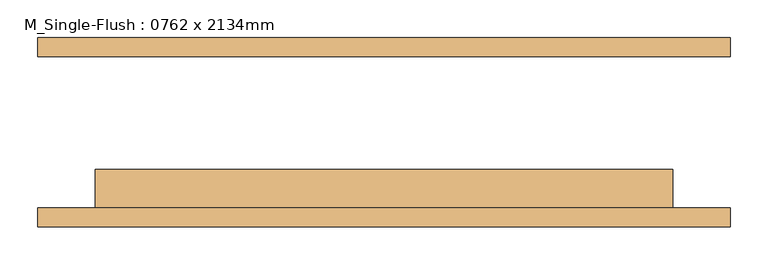
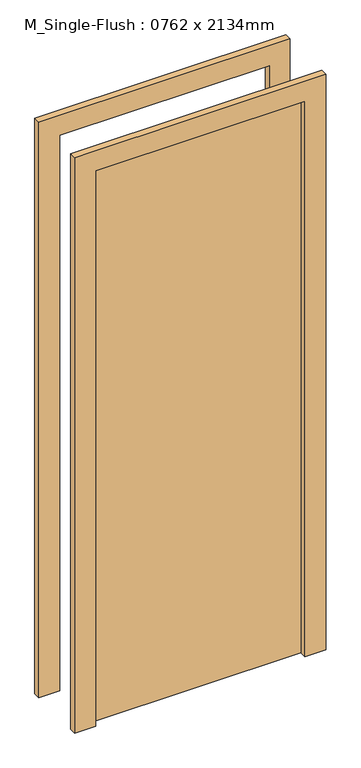
"""IFC4 building model written with IfcOpenShell, lengths in millimetres: door geometry, M_Single-Flush : 0762 x 2134mm."""

from ifc_helpers import new_model, si_unit, frame, origin, origin_with_axes, place, context, project, spatial, polyline, outline, extrude, source, transform, mapped, element, save


def m_single_flush_0762_x_2134mm_f5705a9d(model_context):
    return source(origin(), model_context, "Body", "SweptSolid", [
        extrude(outline(polyline([(2210.0, -457.0), (0.0, -457.0), (0.0, -381.0), (2134.0, -381.0), (2134.0, 381.0), (0.0, 381.0), (0.0, 457.0), (2210.0, 457.0), (2210.0, -457.0)])), frame((0.0, -125.0, 0.0), z_axis=(0.0, 1.0, 0.0), x_axis=(0.0, 0.0, 1.0)), (0.0, 0.0, 1.0), 25.0),
        extrude(outline(polyline([(2210.0, 457.0), (2210.0, -457.0), (0.0, -457.0), (0.0, -381.0), (2134.0, -381.0), (2134.0, 381.0), (0.0, 381.0), (0.0, 457.0), (2210.0, 457.0)])), frame((0.0, 100.0, 0.0), z_axis=(0.0, 1.0, 0.0), x_axis=(0.0, 0.0, 1.0)), (0.0, 0.0, 1.0), 25.0),
        extrude(outline(polyline([(381.0, -49.0), (381.0, -100.0), (-381.0, -100.0), (-381.0, -49.0), (381.0, -49.0)])), origin_with_axes(), (0.0, 0.0, 1.0), 2134.0),
    ])


if __name__ == "__main__":
    model = new_model("IFC4")
    model_context = context("Model", 3, world=origin())
    ifc_project = project(units=[si_unit("LENGTHUNIT", "METRE", prefix="MILLI")], contexts=[model_context])
    site = spatial("IfcSite", under=ifc_project)
    building = spatial("IfcBuilding", under=site)
    placement = place(None, origin())
    m_single_flush_0762_x_2134mm_shape = m_single_flush_0762_x_2134mm_f5705a9d(model_context)
    element("IfcDoor", 1, ObjectType="M_Single-Flush : 0762 x 2134mm", at=placement, inside=building, context=model_context, shape_type="MappedRepresentation", body=[
        mapped(m_single_flush_0762_x_2134mm_shape, transform((0.0, 0.0, 0.0), x_axis=(1.0, 0.0, 0.0), y_axis=(0.0, 1.0, 0.0), z_axis=(0.0, 0.0, 1.0))),
    ])
    save(model, "model.ifc")

# Revit data of these elements
# Type "M_Single-Flush : 0762 x 2134mm"
#   Type Mark = "18"
#   Thickness = 0' - 2.00787"
#   Height = 7' - 0.01575"
#   Trim Projection Ext = 0' - 0.98425"
#   Trim Projection Int = 0' - 0.98425"
#   Trim Width = 0' - 2.99213"
#   Width = 2' - 6"
#   Door Material = Door - Panel
#   Frame Material = Door - Frame
#   Function = (empty or 0)
#   Wall Closure = (empty or 0)
# Element 1 (IfcDoor, "M_Single-Flush : 0762 x 2134mm")
#   Materials on its faces: "Door - Frame", "Door - Panel"
# Materials
#   "Door - Panel": class "Wood", colour RGB 114 82 51, transparency 0
#   "Door - Frame": colour RGB 153 76 43, transparency 0
